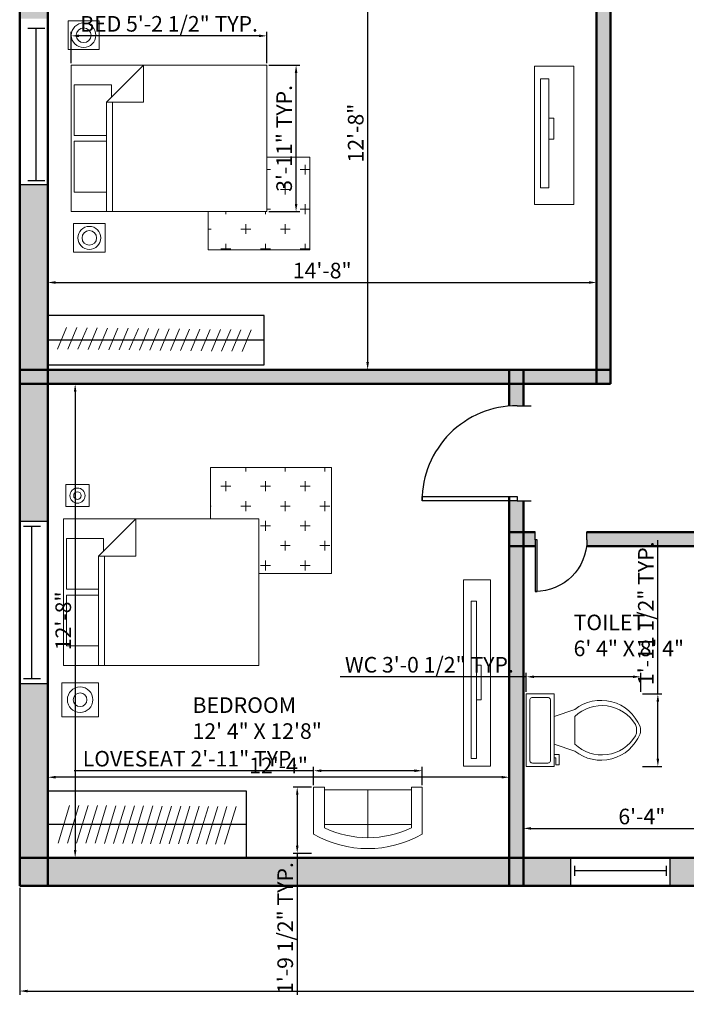
# Model space of a CAD drawing. Units: millimetres. Extents: x 3107 to 3757, y 777 to 1464.
# Tile 1 of 7: x 3110 to 3324, y 824 to 1140. Entities that reach past the tile are written whole.
import ezdxf

# ---------------------------------------------------------------- set-up
doc = ezdxf.new("R2010")
doc.units = ezdxf.units.MM
for name, color, linetype, lineweight in [('A-ANNO-DIMS', 50, 'Continuous', 18), ('A-AREA-IDEN', 160, 'Continuous', 18), ('A-EQPM', 140, 'Continuous', 18), ('A-FLOR-CASE', 140, 'Continuous', 25), ('A-FLOR-CASE-PATT', 140, 'Continuous', 13), ('A-FLOR-FIXT', 140, 'Continuous', 18), ('A-FURN-PATT', 140, 'Continuous', 13), ('A-WALL-PATT', 80, 'Continuous', 13), ('doors', 10, 'Continuous', 25), ('furniture', 140, 'Continuous', 18), ('walls', 80, 'Continuous', 50), ('windows', 30, 'Continuous', 25)]:
    doc.layers.add(name, color=color, linetype=linetype, lineweight=lineweight)
doc.styles.get("Standard").update_dxf_attribs({"font": 'arial.ttf'})
doc.dimstyles.new('ISO-25', dxfattribs={"dimtxt": 5, "dimasz": 2.5, "dimexe": 1.25, "dimexo": 0.625, "dimtad": 1, "dimdec": 0, "dimlunit": 3, "dimtxsty": 'Standard', "dimcen": 2.5, "dimadec": 0, "dimazin": 0, "dimtfac": 1, "dimtdec": 0, "dimtmove": 0, "dimatfit": 3, "dimfxl": 1, "dimarcsym": 0})

# ---------------------------------------------------------------- blocks, each defined once
blk = doc.blocks.new('*U2')
for p, q in [((0, 0), (0, -6)), ((40, 0), (40, -6))]:
    blk.add_line(p, q)
blk.add_lwpolyline([(0, 0), (0, 40), (1.75, 40), (1.75, 0)], close=True)
blk.add_arc((0, 0), 40, 0, 90)
blk = doc.blocks.new('*U4')
for p, q in [((0, 4), (0, 0)), ((36, 4), (36, 0)), ((0, 2), (36, 2))]:
    blk.add_line(p, q)
blk = doc.blocks.new('*U5')
for p, q in [((0, 4), (0, 0)), ((36, 4), (36, 0)), ((0, 2), (36, 2))]:
    blk.add_line(p, q)
blk = doc.blocks.new('Toilet - top')
for p, q in [((9.5, -6), (9.5, -2)), ((-10, -8.5), (-8, -8.5)), ((-10, -9.5), (-10, -8.5)), ((-8, -8.5), (-8, -8)), ((-7, -8), (-7, -9.5)), ((-4, -8), (-6, -14)), ((4, -8), (6, -14)), ((-7, -9.5), (-10, -9.5)), ((4, -14), (-4, -14))]:
    blk.add_line(p, q)
blk.add_lwpolyline([(10.5, -8), (10.5, 0), (-10.5, 0), (-10.5, -8)], close=True)
for points in [[(-9.5, -2), (-9.5, -6)], [(8.5, -1), (-8.5, -1)], [(-8.5, -7), (8.5, -7)]]:
    blk.add_lwpolyline(points)
for centre, radius, start, end in [((-8.62, -1.88), 0.884, 81.8699, 188.1301), ((8.62, -1.88), 0.884, 351.8699, 98.1301), ((-8.62, -6.12), 0.884, 171.8699, 278.1301), ((8.62, -6.12), 0.884, 261.8699, 8.1301), ((3.52, -21.58), 12.17, 141.4691, 247.9714), ((4.2, -21.82), 11.33, 136.3677, 238.9468), ((-3.52, -21.58), 12.17, 292.0284, 38.5307), ((-4.2, -21.82), 11.33, 301.053, 43.6321), ((0, -27.88), 4, 245.7318, 294.2682), ((0, -29), 4, 254.8605, 285.1395)]:
    blk.add_arc(centre, radius, start, end)
blk = doc.blocks.new('Bed - Queen')
for p, q in [((0, -80.00003), (0, 0)), ((0, 0), (59.99999, 0)), ((59.99999, 0), (59.99999, -80.00003)), ((7.99999, -1.2), (28.79998, -1.2)), ((7.99999, -14.4), (7.99999, -1.2)), ((28.79998, -1.2), (28.79998, -14.4)), ((31.19999, -1.2), (51.99999, -1.2)), ((31.19999, -14.4), (31.19999, -1.2)), ((51.99999, -1.2), (51.99999, -16.4)), ((0, -14.4), (44.8, -14.4)), ((59.99999, -29.6), (44.8, -14.4)), ((44.8, -14.4), (44.8, -29.6)), ((44.8, -16.8), (0, -16.8)), ((51.99999, -16.4), (46.79936, -16.4)), ((44.8, -29.6), (59.99999, -29.6)), ((59.99999, -80.00003), (0, -80.00003))]:
    blk.add_line(p, q)
blk = doc.blocks.new('Sofa - Roundback Loveseat 5 ft.')
for p, q in [((0, -32.44198), (0, -5.99998)), ((-24, -33.99998), (-24, -11.46958)), ((-23.9998, -13.38178), (23.99986, -13.38178)), ((24.00004, -33.99998), (24.00004, -11.46958)), ((-24, -32.44198), (24.00004, -32.44198))]:
    blk.add_line(p, q)
for points in [[(-24, -33.99998), (-30, -33.99998), (-30, -7.99998)], [(30.00004, -7.99998), (30.00004, -33.99998), (24.00004, -33.99998)]]:
    blk.add_lwpolyline(points)
for centre, radius, start, end in [((0, -60.24998), 60.24998, 60.13715, 119.8628), ((0, -61.38438), 55.38444, 64.32083, 115.6792)]:
    blk.add_arc(centre, radius, start, end)
blk = doc.blocks.new('*D32')
at = {"layer": 'A-ANNO-DIMS', "color": 0, "lineweight": -2, "transparency": 16777216}
for p, q in [((3119.47, 1056.03), (3119.47, 1054.74)), ((3121.97, 1055.99), (3292.97, 1055.99)), ((3295.47, 1056.03), (3295.47, 1054.74))]:
    blk.add_line(p, q, dxfattribs=at)
at = {"layer": 'A-ANNO-DIMS', "color": 0, "transparency": 16777216}
for points in [[(3121.97, 1056.41), (3121.97, 1055.57), (3119.47, 1055.99)], [(3292.97, 1056.41), (3292.97, 1055.57), (3295.47, 1055.99)]]:
    blk.add_solid(points, dxfattribs=at)
at = {"layer": 'Defpoints', "color": 0, "transparency": 16777216}
for p in [(3119.47, 1056.66), (3295.47, 1056.66), (3295.47, 1055.99)]:
    blk.add_point(p, dxfattribs=at)
at = {"layer": 'A-ANNO-DIMS', "color": 0, "transparency": 16777216, "insert": (3207.47, 1059.17), "char_height": 5, "attachment_point": 5}
blk.add_mtext('14\'-8"', dxfattribs=at)
blk = doc.blocks.new('*D33')
at = {"layer": 'A-ANNO-DIMS', "color": 0, "lineweight": -2, "transparency": 16777216}
for p, q in [((3221.28, 1179.93), (3223.29, 1179.93)), ((3222.04, 1177.43), (3222.04, 1030.43)), ((3221.28, 1027.93), (3223.29, 1027.93))]:
    blk.add_line(p, q, dxfattribs=at)
at = {"layer": 'A-ANNO-DIMS', "color": 0, "transparency": 16777216}
for points in [[(3221.62, 1177.43), (3222.45, 1177.43), (3222.04, 1179.93)], [(3221.62, 1030.43), (3222.45, 1030.43), (3222.04, 1027.93)]]:
    blk.add_solid(points, dxfattribs=at)
at = {"layer": 'Defpoints', "color": 0, "transparency": 16777216}
for p in [(3220.65, 1179.93), (3220.65, 1027.93), (3222.04, 1027.93)]:
    blk.add_point(p, dxfattribs=at)
at = {"layer": 'A-ANNO-DIMS', "color": 0, "transparency": 16777216, "insert": (3218.86, 1103.93), "char_height": 5, "attachment_point": 5, "rotation": 90}
blk.add_mtext('12\'-8"', dxfattribs=at)
blk = doc.blocks.new('*D34')
at = {"layer": 'A-ANNO-DIMS', "color": 0, "lineweight": -2, "transparency": 16777216}
for p, q in [((3119.47, 896.29), (3119.47, 898.5)), ((3264.97, 897.25), (3121.97, 897.25)), ((3267.47, 896.29), (3267.47, 898.5))]:
    blk.add_line(p, q, dxfattribs=at)
at = {"layer": 'A-ANNO-DIMS', "color": 0, "transparency": 16777216}
for points in [[(3121.97, 897.67), (3121.97, 896.84), (3119.47, 897.25)], [(3264.97, 897.67), (3264.97, 896.84), (3267.47, 897.25)]]:
    blk.add_solid(points, dxfattribs=at)
at = {"layer": 'Defpoints', "color": 0, "transparency": 16777216}
for p in [(3119.47, 897.25), (3119.47, 895.66), (3267.47, 895.66)]:
    blk.add_point(p, dxfattribs=at)
at = {"layer": 'A-ANNO-DIMS', "color": 0, "transparency": 16777216, "insert": (3193.47, 900.39), "char_height": 5, "attachment_point": 5}
blk.add_mtext('12\'-4"', dxfattribs=at)
blk = doc.blocks.new('*D35')
at = {"layer": 'A-ANNO-DIMS', "color": 0, "lineweight": -2, "transparency": 16777216}
for p, q in [((3126.83, 1023.43), (3129.5, 1023.43)), ((3128.25, 1020.93), (3128.25, 873.93)), ((3126.83, 871.43), (3129.5, 871.43))]:
    blk.add_line(p, q, dxfattribs=at)
at = {"layer": 'A-ANNO-DIMS', "color": 0, "transparency": 16777216}
for points in [[(3127.84, 1020.93), (3128.67, 1020.93), (3128.25, 1023.43)], [(3127.84, 873.93), (3128.67, 873.93), (3128.25, 871.43)]]:
    blk.add_solid(points, dxfattribs=at)
at = {"layer": 'Defpoints', "color": 0, "transparency": 16777216}
for p in [(3126.21, 1023.43), (3126.21, 871.43), (3128.25, 871.43)]:
    blk.add_point(p, dxfattribs=at)
at = {"layer": 'A-ANNO-DIMS', "color": 0, "transparency": 16777216, "insert": (3125.08, 947.43), "char_height": 5, "attachment_point": 5, "rotation": 90}
blk.add_mtext('12\'-8"', dxfattribs=at)
blk = doc.blocks.new('*D37')
at = {"layer": 'A-ANNO-DIMS', "color": 0, "lineweight": -2, "transparency": 16777216}
for p, q in [((3271.97, 881.46), (3271.97, 882.08)), ((3347.97, 881.46), (3347.97, 882.08)), ((3274.47, 880.83), (3345.47, 880.83))]:
    blk.add_line(p, q, dxfattribs=at)
at = {"layer": 'A-ANNO-DIMS', "color": 0, "transparency": 16777216}
for points in [[(3274.47, 881.25), (3274.47, 880.41), (3271.97, 880.83)], [(3345.47, 881.25), (3345.47, 880.41), (3347.97, 880.83)]]:
    blk.add_solid(points, dxfattribs=at)
at = {"layer": 'Defpoints', "color": 0, "transparency": 16777216}
for p in [(3271.97, 880.83), (3347.97, 880.83), (3347.97, 880.83)]:
    blk.add_point(p, dxfattribs=at)
at = {"layer": 'A-ANNO-DIMS', "color": 0, "transparency": 16777216, "insert": (3309.97, 884.01), "char_height": 5, "attachment_point": 5}
blk.add_mtext('6\'-4"', dxfattribs=at)
blk = doc.blocks.new('*D49')
at = {"layer": 'A-ANNO-DIMS', "color": 0, "lineweight": -2, "transparency": 16777216}
for p, q in [((3127.01, 1126.35), (3127.01, 1136.38)), ((3187.19, 1135.13), (3129.51, 1135.13)), ((3189.69, 1126.35), (3189.69, 1136.38))]:
    blk.add_line(p, q, dxfattribs=at)
at = {"layer": 'A-ANNO-DIMS', "color": 0, "transparency": 16777216}
for points in [[(3129.51, 1135.55), (3129.51, 1134.71), (3127.01, 1135.13)], [(3187.19, 1135.55), (3187.19, 1134.71), (3189.69, 1135.13)]]:
    blk.add_solid(points, dxfattribs=at)
at = {"layer": 'Defpoints', "color": 0, "transparency": 16777216}
for p in [(3127.01, 1135.13), (3127.01, 1125.73), (3189.69, 1125.73)]:
    blk.add_point(p, dxfattribs=at)
at = {"layer": 'A-ANNO-DIMS', "color": 0, "transparency": 16777216, "insert": (3158.35, 1138.34), "char_height": 5, "attachment_point": 5}
blk.add_mtext('BED 5\'-2 1/2" TYP.', dxfattribs=at)
blk = doc.blocks.new('*D50')
at = {"layer": 'A-ANNO-DIMS', "color": 0, "lineweight": -2, "transparency": 16777216}
for p, q in [((3190.32, 1125.73), (3200.34, 1125.73)), ((3199.09, 1081.22), (3199.09, 1123.23)), ((3190.32, 1078.72), (3200.34, 1078.72))]:
    blk.add_line(p, q, dxfattribs=at)
at = {"layer": 'A-ANNO-DIMS', "color": 0, "transparency": 16777216}
for points in [[(3198.68, 1123.23), (3199.51, 1123.23), (3199.09, 1125.73)], [(3198.68, 1081.22), (3199.51, 1081.22), (3199.09, 1078.72)]]:
    blk.add_solid(points, dxfattribs=at)
at = {"layer": 'Defpoints', "color": 0, "transparency": 16777216}
for p in [(3189.69, 1125.73), (3199.09, 1125.73), (3189.69, 1078.72)]:
    blk.add_point(p, dxfattribs=at)
at = {"layer": 'A-ANNO-DIMS', "color": 0, "transparency": 16777216, "insert": (3195.91, 1102.22), "char_height": 5, "attachment_point": 5, "rotation": 90}
blk.add_mtext('3\'-11" TYP.', dxfattribs=at)
blk = doc.blocks.new('*D51')
at = {"layer": 'A-ANNO-DIMS', "color": 0, "lineweight": -2, "transparency": 16777216}
for p, q in [((3272.92, 929.48), (3213.26, 929.48)), ((3272.92, 924.6), (3272.92, 930.73)), ((3307.1, 929.48), (3275.42, 929.48)), ((3309.6, 924.6), (3309.6, 930.73))]:
    blk.add_line(p, q, dxfattribs=at)
at = {"layer": 'A-ANNO-DIMS', "color": 0, "transparency": 16777216}
for points in [[(3275.42, 929.89), (3275.42, 929.06), (3272.92, 929.48)], [(3307.1, 929.89), (3307.1, 929.06), (3309.6, 929.48)]]:
    blk.add_solid(points, dxfattribs=at)
at = {"layer": 'Defpoints', "color": 0, "transparency": 16777216}
for p in [(3272.92, 929.48), (3272.92, 923.97), (3309.6, 923.97)]:
    blk.add_point(p, dxfattribs=at)
at = {"layer": 'A-ANNO-DIMS', "color": 0, "transparency": 16777216, "insert": (3241.84, 932.69), "char_height": 5, "attachment_point": 5}
blk.add_mtext('WC 3\'-0 1/2" TYP.', dxfattribs=at)
blk = doc.blocks.new('*D52')
at = {"layer": 'A-ANNO-DIMS', "color": 0, "lineweight": -2, "transparency": 16777216}
for p, q in [((3315.1, 923.97), (3315.1, 973.27)), ((3310.22, 923.97), (3316.35, 923.97)), ((3315.1, 903.16), (3315.1, 921.47)), ((3310.22, 900.66), (3316.35, 900.66))]:
    blk.add_line(p, q, dxfattribs=at)
at = {"layer": 'A-ANNO-DIMS', "color": 0, "transparency": 16777216}
for points in [[(3314.69, 921.47), (3315.52, 921.47), (3315.1, 923.97)], [(3314.69, 903.16), (3315.52, 903.16), (3315.1, 900.66)]]:
    blk.add_solid(points, dxfattribs=at)
at = {"layer": 'Defpoints', "color": 0, "transparency": 16777216}
for p in [(3309.6, 923.97), (3315.1, 923.97), (3309.6, 900.66)]:
    blk.add_point(p, dxfattribs=at)
at = {"layer": 'A-ANNO-DIMS', "color": 0, "transparency": 16777216, "insert": (3311.89, 949.87), "char_height": 5, "attachment_point": 5, "rotation": 90}
blk.add_mtext('1\'-11 1/2" TYP.', dxfattribs=at)
blk = doc.blocks.new('*D59')
at = {"layer": 'A-ANNO-DIMS', "color": 0, "lineweight": -2, "transparency": 16777216}
for p, q in [((3204.69, 894.74), (3204.69, 900.59)), ((3239.55, 894.74), (3239.55, 900.59)), ((3204.69, 899.34), (3127.98, 899.34)), ((3237.05, 899.34), (3207.19, 899.34))]:
    blk.add_line(p, q, dxfattribs=at)
at = {"layer": 'A-ANNO-DIMS', "color": 0, "transparency": 16777216}
for points in [[(3207.19, 899.76), (3207.19, 898.92), (3204.69, 899.34)], [(3237.05, 899.76), (3237.05, 898.92), (3239.55, 899.34)]]:
    blk.add_solid(points, dxfattribs=at)
at = {"layer": 'Defpoints', "color": 0, "transparency": 16777216}
for p in [(3204.69, 899.34), (3204.69, 894.11), (3239.55, 894.11)]:
    blk.add_point(p, dxfattribs=at)
at = {"layer": 'A-ANNO-DIMS', "color": 0, "transparency": 16777216, "insert": (3165.09, 902.55), "char_height": 5, "attachment_point": 5, "rotation": 360}
blk.add_mtext('LOVESEAT 2\'-11" TYP.', dxfattribs=at)
blk = doc.blocks.new('*D60')
at = {"layer": 'A-ANNO-DIMS', "color": 0, "lineweight": -2, "transparency": 16777216}
for p, q in [((3204.07, 894.11), (3198.21, 894.11)), ((3199.46, 891.61), (3199.46, 875.31)), ((3204.07, 872.81), (3198.21, 872.81)), ((3199.46, 872.81), (3199.46, 827.4))]:
    blk.add_line(p, q, dxfattribs=at)
at = {"layer": 'A-ANNO-DIMS', "color": 0, "transparency": 16777216}
for points in [[(3199.05, 891.61), (3199.88, 891.61), (3199.46, 894.11)], [(3199.05, 875.31), (3199.88, 875.31), (3199.46, 872.81)]]:
    blk.add_solid(points, dxfattribs=at)
at = {"layer": 'Defpoints', "color": 0, "transparency": 16777216}
for p in [(3204.69, 894.11), (3199.46, 872.81), (3204.69, 872.81)]:
    blk.add_point(p, dxfattribs=at)
at = {"layer": 'A-ANNO-DIMS', "color": 0, "transparency": 16777216, "insert": (3196.25, 848.86), "char_height": 5, "attachment_point": 5, "rotation": 90}
blk.add_mtext('1\'-9 1/2" TYP.', dxfattribs=at)
blk = doc.blocks.new('*D69')
at = {"layer": 'A-ANNO-DIMS', "color": 0, "lineweight": -2, "transparency": 16777216}
for p, q in [((3110.47, 861.8), (3110.47, 827.39)), ((3721.97, 861.8), (3721.97, 827.39)), ((3112.97, 828.64), (3719.47, 828.64))]:
    blk.add_line(p, q, dxfattribs=at)
at = {"layer": 'A-ANNO-DIMS', "color": 0, "transparency": 16777216}
for points in [[(3112.97, 829.06), (3112.97, 828.22), (3110.47, 828.64)], [(3719.47, 829.06), (3719.47, 828.22), (3721.97, 828.64)]]:
    blk.add_solid(points, dxfattribs=at)
at = {"layer": 'Defpoints', "color": 0, "transparency": 16777216}
for p in [(3110.47, 862.43), (3721.97, 862.43), (3721.97, 828.64)]:
    blk.add_point(p, dxfattribs=at)
at = {"layer": 'A-ANNO-DIMS', "color": 0, "transparency": 16777216, "insert": (3416.22, 831.85), "char_height": 5, "attachment_point": 5}
blk.add_mtext('50\'-11 1/2"', dxfattribs=at)

msp = doc.modelspace()

# ---------------------------------------------------------------- hatches: boundary and pattern name
at = {"layer": 'A-FLOR-CASE-PATT'}
h = msp.add_hatch(dxfattribs=at)
h.set_pattern_fill('ANSI31', color=256, scale=0.960855, angle=22.188, style=0)
h.paths.add_polyline_path([(3120.7, 1034.66), (3123.99, 1034.62), (3130.57, 1034.53), (3166.78, 1034.07), (3176.66, 1033.94), (3183.24, 1033.85), (3186.14, 1040.76), (3123.6, 1041.57)])
h = msp.add_hatch(dxfattribs=at)
h.set_pattern_fill('ANSI31', color=256, scale=0.895394, angle=27.967, style=0)
h.paths.add_polyline_path([(3120.31, 876.16), (3126.24, 876.12), (3155.91, 875.91), (3161.84, 875.87), (3176.68, 875.76), (3180.38, 887.84), (3150.71, 888.05), (3147.74, 888.07), (3124.01, 888.24)])
at = {"layer": 'A-FURN-PATT'}
h = msp.add_hatch(dxfattribs=at)
h.set_pattern_fill('CROSS', color=256)
h.paths.add_polyline_path([(3203.54, 1096.17), (3189.69, 1096.17), (3189.69, 1078.72), (3170.92, 1078.72), (3170.92, 1066.5), (3203.54, 1066.5)])
h = msp.add_hatch(dxfattribs=at)
h.set_pattern_fill('CROSS', color=256)
h.paths.add_polyline_path([(3171.7, 996.6), (3171.7, 980.14), (3187.18, 980.14), (3187.18, 962.6), (3210.42, 962.6), (3210.42, 996.6)])
at = {"layer": 'A-WALL-PATT'}
h = msp.add_hatch(color=256, dxfattribs=at)
h.dxf.hatch_style = 1
h.paths.add_polyline_path([(3119.47, 1087.39), (3110.47, 1087.39), (3110.47, 1027.93), (3119.47, 1027.93)])
h.paths.add_polyline_path([(3119.47, 1027.93), (3110.47, 1027.93), (3110.47, 1023.43), (3119.47, 1023.43)])
h.paths.add_polyline_path([(3267.47, 1027.93), (3119.47, 1027.93), (3119.47, 1023.43), (3267.47, 1023.43)])
h.paths.add_polyline_path([(3119.47, 1023.43), (3110.47, 1023.43), (3110.47, 979.44), (3119.47, 979.44)])
h.paths.add_polyline_path([(3299.97, 1179.93), (3295.47, 1179.93), (3295.47, 1027.93), (3299.97, 1027.93)])
h.paths.add_polyline_path([(3295.47, 1027.93), (3271.97, 1027.93), (3271.97, 1023.43), (3295.47, 1023.43)])
h.paths.add_polyline_path([(3271.97, 1027.93), (3267.47, 1027.93), (3267.47, 1023.43), (3271.97, 1023.43)])
h.paths.add_polyline_path([(3299.97, 1027.93), (3295.47, 1027.93), (3295.47, 1023.43), (3299.97, 1023.43)])
h.paths.add_polyline_path([(3299.97, 1184.43), (3295.47, 1184.43), (3295.47, 1179.93), (3299.97, 1179.93)])
h.paths.add_polyline_path([(3295.47, 1184.43), (3288.38, 1184.43), (3288.38, 1182.47), (3288.38, 1179.93), (3295.47, 1179.93)])
h.paths.add_polyline_path([(3352.47, 1179.93), (3347.97, 1179.93), (3347.97, 1027.93), (3352.47, 1027.93)])
h.paths.add_polyline_path([(3352.47, 1184.43), (3347.97, 1184.43), (3347.97, 1179.93), (3352.47, 1179.93)])
h.paths.add_polyline_path([(3464.47, 1184.43), (3352.47, 1184.43), (3352.47, 1179.93), (3464.47, 1179.93)])
h.paths.add_polyline_path([(3468.97, 1288.93), (3464.47, 1288.93), (3464.47, 1184.43), (3468.97, 1184.43)])
h.paths.add_polyline_path([(3468.97, 1184.43), (3464.47, 1184.43), (3464.47, 1179.93), (3468.97, 1179.93)])
h.paths.add_polyline_path([(3195.97, 1248.43), (3191.47, 1248.43), (3191.47, 1184.43), (3195.97, 1184.43)])
h.paths.add_polyline_path([(3195.97, 1184.43), (3191.47, 1184.43), (3191.47, 1179.93), (3195.97, 1179.93)])
h.paths.add_polyline_path([(3191.47, 1184.43), (3183.28, 1184.43), (3183.28, 1181.58), (3183.28, 1179.93), (3191.47, 1179.93)])
h.paths.add_polyline_path([(3243.97, 1184.43), (3195.97, 1184.43), (3195.97, 1179.93), (3243.97, 1179.93)])
h.paths.add_polyline_path([(3257.91, 1182.47), (3257.91, 1184.43), (3248.47, 1184.43), (3248.47, 1179.93), (3258.02, 1179.93, -0.020891)])
h.paths.add_polyline_path([(3248.47, 1184.43), (3243.97, 1184.43), (3243.97, 1179.93), (3248.47, 1179.93)])
h.paths.add_polyline_path([(3248.47, 1189.24), (3247.51, 1189.24), (3243.97, 1189.24), (3243.97, 1184.43), (3248.47, 1184.43)])
h.paths.add_polyline_path([(3166.87, 1184.43), (3119.47, 1184.43), (3119.47, 1179.93), (3166.63, 1179.93), (3166.63, 1181.58, -0.042981)])
h.paths.add_polyline_path([(3119.47, 1184.43), (3110.47, 1184.43), (3110.47, 1179.93), (3119.47, 1179.93)])
h.paths.add_polyline_path([(3119.47, 1248.43), (3110.47, 1248.43), (3110.47, 1184.43), (3119.47, 1184.43)])
h.paths.add_polyline_path([(3119.47, 1179.93), (3110.47, 1179.93), (3110.47, 1140.65), (3119.47, 1140.65)])
h.paths.add_polyline_path([(3119.47, 1288.93), (3110.47, 1288.93), (3110.47, 1252.93), (3119.47, 1252.93)])
h.paths.add_polyline_path([(3119.47, 1252.93), (3110.47, 1252.93), (3110.47, 1248.43), (3119.47, 1248.43)])
h.paths.add_polyline_path([(3191.47, 1252.93), (3119.47, 1252.93), (3119.47, 1248.43), (3191.47, 1248.43)])
h.paths.add_polyline_path([(3195.97, 1288.93), (3191.47, 1288.93), (3191.47, 1252.93), (3195.97, 1252.93)])
h.paths.add_polyline_path([(3195.97, 1252.93), (3191.47, 1252.93), (3191.47, 1248.43), (3195.97, 1248.43)])
h.paths.add_polyline_path([(3248.47, 1293.43), (3243.97, 1293.43), (3243.97, 1288.93), (3248.47, 1288.93)])
h.paths.add_polyline_path([(3243.97, 1293.43), (3195.97, 1293.43), (3195.97, 1288.93), (3243.97, 1288.93)])
h.paths.add_polyline_path([(3303.47, 1293.43), (3248.47, 1293.43), (3248.47, 1288.93), (3303.47, 1288.93)])
h.paths.add_polyline_path([(3248.47, 1288.93), (3243.97, 1288.93), (3243.97, 1205.51, -0.053712), (3247.51, 1205.89), (3248.47, 1205.89)])
h.paths.add_polyline_path([(3191.47, 1293.43), (3119.47, 1293.43), (3119.47, 1288.93), (3191.47, 1288.93)])
h.paths.add_polyline_path([(3119.47, 1293.43), (3110.47, 1293.43), (3110.47, 1288.93), (3119.47, 1288.93)])
h.paths.add_polyline_path([(3119.47, 1322.96, -0.065064), (3111.64, 1321.93), (3110.47, 1321.93), (3110.47, 1293.43), (3119.47, 1293.43)])
h.paths.add_polyline_path([(3195.97, 1293.43), (3191.47, 1293.43), (3191.47, 1288.93), (3195.97, 1288.93)])
h.paths.add_polyline_path([(3119.47, 1450.43), (3110.47, 1450.43), (3110.47, 1441.43), (3119.47, 1441.43)])
h.paths.add_polyline_path([(3119.47, 1441.43), (3110.47, 1441.43), (3110.47, 1352.4), (3111.64, 1352.4), (3119.47, 1352.4)])
h.paths.add_polyline_path([(3176.58, 1450.43), (3119.47, 1450.43), (3119.47, 1441.43), (3176.58, 1441.43)])
h.paths.add_polyline_path([(3323.19, 1450.43), (3307.97, 1450.43), (3307.97, 1441.43), (3323.19, 1441.43)])
h.paths.add_polyline_path([(3307.97, 1450.43), (3303.47, 1450.43), (3303.47, 1441.43), (3307.97, 1441.43)])
h.paths.add_polyline_path([(3303.47, 1450.43), (3229.4, 1450.43), (3229.4, 1441.43), (3303.47, 1441.43)])
h.paths.add_polyline_path([(3307.97, 1441.43), (3303.47, 1441.43), (3303.47, 1363.43), (3307.97, 1363.43)])
h.paths.add_polyline_path([(3307.97, 1363.43), (3303.47, 1363.43), (3303.47, 1358.93), (3307.97, 1358.93)])
h.paths.add_polyline_path([(3307.97, 1358.93), (3303.47, 1358.93), (3303.47, 1342.3), (3305.5, 1342.3, -0.037178), (3307.97, 1342.12)])
h.paths.add_polyline_path([(3379.97, 1363.43), (3307.97, 1363.43), (3307.97, 1358.93), (3379.97, 1358.93)])
h.paths.add_polyline_path([(3384.47, 1393.61), (3383.04, 1393.61), (3379.97, 1393.61), (3379.97, 1363.43), (3384.47, 1363.43)])
h.paths.add_polyline_path([(3384.47, 1363.43), (3379.97, 1363.43), (3379.97, 1358.93), (3384.47, 1358.93)])
h.paths.add_polyline_path([(3384.47, 1358.93), (3379.97, 1358.93), (3379.97, 1293.43), (3384.47, 1293.43)])
h.paths.add_polyline_path([(3384.47, 1441.43), (3379.97, 1441.43), (3379.97, 1409.98, -0.046389), (3383.04, 1410.27), (3384.47, 1410.27)])
h.paths.add_polyline_path([(3384.47, 1450.43), (3379.97, 1450.43), (3379.97, 1441.43), (3384.47, 1441.43)])
h.paths.add_polyline_path([(3379.97, 1450.43), (3357.18, 1450.43), (3357.18, 1441.43), (3379.97, 1441.43)])
h.paths.add_polyline_path([(3432.79, 1450.43), (3384.47, 1450.43), (3384.47, 1441.43), (3432.79, 1441.43)])
h.paths.add_polyline_path([(3540.47, 1450.43), (3484.18, 1450.43), (3484.18, 1441.43), (3540.47, 1441.43)])
h.paths.add_polyline_path([(3544.97, 1450.43), (3540.47, 1450.43), (3540.47, 1441.43), (3544.97, 1441.43)])
h.paths.add_polyline_path([(3544.97, 1441.43), (3540.47, 1441.43), (3540.47, 1293.43), (3544.97, 1293.43)])
h.paths.add_polyline_path([(3590.83, 1450.43), (3544.97, 1450.43), (3544.97, 1441.43), (3590.83, 1441.43)])
h.paths.add_polyline_path([(3712.97, 1450.43), (3645.62, 1450.43), (3645.62, 1441.43), (3712.97, 1441.43)])
h.paths.add_polyline_path([(3721.97, 1441.43), (3712.97, 1441.43), (3712.97, 1288.93), (3712.97, 1184.43), (3721.97, 1184.43), (3721.97, 1288.93)])
h.paths.add_polyline_path([(3721.97, 1450.43), (3712.97, 1450.43), (3712.97, 1441.43), (3721.97, 1441.43)])
h.paths.add_polyline_path([(3712.97, 1184.43), (3658.24, 1184.43), (3658.24, 1183.15), (3658.24, 1179.93), (3712.97, 1179.93)])
h.paths.add_polyline_path([(3721.97, 1184.43), (3712.97, 1184.43), (3712.97, 1179.93), (3721.97, 1179.93)])
h.paths.add_polyline_path([(3597.32, 1183.15), (3597.32, 1184.43), (3544.97, 1184.43), (3544.97, 1179.93), (3597.32, 1179.93)])
h.paths.add_polyline_path([(3544.97, 1184.43), (3540.47, 1184.43), (3540.47, 1179.93), (3544.97, 1179.93)])
h.paths.add_polyline_path([(3544.97, 1179.93), (3540.47, 1179.93), (3540.47, 1143.69), (3543.65, 1143.69), (3544.97, 1143.69)])
h.paths.add_polyline_path([(3721.97, 1179.93), (3712.97, 1179.93), (3712.97, 1006.22), (3712.97, 871.43), (3721.97, 871.43), (3721.97, 1006.22)])
h.paths.add_polyline_path([(3468.97, 1293.43), (3464.47, 1293.43), (3464.47, 1288.93), (3468.97, 1288.93)])
h.paths.add_polyline_path([(3540.47, 1293.43), (3468.97, 1293.43), (3468.97, 1288.93), (3540.47, 1288.93)])
h.paths.add_polyline_path([(3544.97, 1293.43), (3540.47, 1293.43), (3540.47, 1288.93), (3544.97, 1288.93)])
h.paths.add_polyline_path([(3464.47, 1293.43), (3417.83, 1293.43, -0.015057), (3417.88, 1291.6), (3417.88, 1288.93), (3464.47, 1288.93)])
h.paths.add_polyline_path([(3379.97, 1293.43), (3307.97, 1293.43), (3307.97, 1288.93), (3379.97, 1288.93)])
h.paths.add_polyline_path([(3307.97, 1325.65), (3305.5, 1325.65), (3303.47, 1325.65), (3303.47, 1293.43), (3307.97, 1293.43)])
h.paths.add_polyline_path([(3307.97, 1293.43), (3303.47, 1293.43), (3303.47, 1288.93), (3307.97, 1288.93)])
h.paths.add_polyline_path([(3384.47, 1293.43), (3379.97, 1293.43), (3379.97, 1288.93), (3384.47, 1288.93)])
h.paths.add_polyline_path([(3387.42, 1291.6), (3387.42, 1293.43), (3384.47, 1293.43), (3384.47, 1288.93), (3387.42, 1288.93)])
h.paths.add_polyline_path([(3119.47, 927.28), (3110.47, 927.28), (3110.47, 871.43), (3119.47, 871.43)])
h.paths.add_polyline_path([(3119.47, 871.43), (3110.47, 871.43), (3110.47, 862.43), (3119.47, 862.43)])
h.paths.add_polyline_path([(3267.47, 871.43), (3119.47, 871.43), (3119.47, 862.43), (3267.47, 862.43)])
h.paths.add_polyline_path([(3271.97, 971.43), (3267.47, 971.43), (3267.47, 871.43), (3271.97, 871.43)])
h.paths.add_polyline_path([(3271.97, 871.43), (3267.47, 871.43), (3267.47, 862.43), (3271.97, 862.43)])
h.paths.add_polyline_path([(3287.13, 871.43), (3271.97, 871.43), (3271.97, 862.43), (3287.13, 862.43)])
h.paths.add_polyline_path([(3347.97, 871.43), (3318.96, 871.43), (3318.96, 862.43), (3347.97, 862.43)])
h.paths.add_polyline_path([(3352.47, 971.43), (3347.97, 971.43), (3347.97, 871.43), (3352.47, 871.43)])
h.paths.add_polyline_path([(3352.47, 871.43), (3347.97, 871.43), (3347.97, 862.43), (3352.47, 862.43)])
h.paths.add_polyline_path([(3375.96, 871.43), (3352.47, 871.43), (3352.47, 862.43), (3375.96, 862.43)])
h.paths.add_polyline_path([(3352.47, 975.93), (3347.97, 975.93), (3347.97, 971.43), (3352.47, 971.43)])
h.paths.add_polyline_path([(3352.47, 986.27, -0.01722), (3350.37, 986.2), (3347.97, 986.2), (3347.97, 975.93), (3352.47, 975.93)])
h.paths.add_polyline_path([(3347.97, 975.93), (3292.38, 975.93), (3292.38, 973.47, -0.030785), (3292.25, 971.43), (3347.97, 971.43)])
h.paths.add_polyline_path([(3271.97, 985.98), (3269.95, 985.98), (3267.47, 985.98), (3267.47, 975.93), (3271.97, 975.93)])
h.paths.add_polyline_path([(3271.97, 975.93), (3267.47, 975.93), (3267.47, 971.43), (3271.97, 971.43)])
h.paths.add_polyline_path([(3275.72, 975.93), (3271.97, 975.93), (3271.97, 971.43), (3275.72, 971.43), (3275.72, 973.47)])
h.paths.add_polyline_path([(3271.97, 1023.43), (3267.47, 1023.43), (3267.47, 1016.34, -0.020418), (3269.95, 1016.44), (3271.97, 1016.44)])
h.paths.add_polyline_path([(3352.47, 1023.43), (3347.97, 1023.43), (3347.97, 1016.67), (3350.37, 1016.67), (3352.47, 1016.67)])
h.paths.add_polyline_path([(3352.47, 1027.93), (3347.97, 1027.93), (3347.97, 1023.43), (3352.47, 1023.43)])
h.paths.add_polyline_path([(3476.47, 1027.93), (3352.47, 1027.93), (3352.47, 1023.43), (3476.47, 1023.43)])
h.paths.add_polyline_path([(3540.47, 1027.93), (3480.97, 1027.93), (3480.97, 1023.43), (3540.47, 1023.43)])
h.paths.add_polyline_path([(3480.97, 1027.93), (3476.47, 1027.93), (3476.47, 1023.43), (3480.97, 1023.43)])
h.paths.add_polyline_path([(3480.97, 1023.43), (3476.47, 1023.43), (3476.47, 871.43), (3480.97, 871.43)])
h.paths.add_polyline_path([(3476.47, 871.43), (3429.88, 871.43), (3429.88, 862.43), (3476.47, 862.43)])
h.paths.add_polyline_path([(3480.97, 871.43), (3476.47, 871.43), (3476.47, 862.43), (3480.97, 862.43)])
h.paths.add_polyline_path([(3493.81, 871.43), (3480.97, 871.43), (3480.97, 862.43), (3493.81, 862.43)])
h.paths.add_polyline_path([(3712.97, 871.43), (3525.61, 871.43), (3525.61, 862.43), (3712.97, 862.43)])
h.paths.add_polyline_path([(3721.97, 871.43), (3712.97, 871.43), (3712.97, 862.43), (3721.97, 862.43)])

# ---------------------------------------------------------------- linework, layer by layer
at = {"layer": 'A-EQPM'}
for points in [[(3275.55, 1125.39), (3288.18, 1125.39), (3288.18, 1081.06), (3275.55, 1081.06)], [(3277.46, 1121.35), (3280.17, 1121.35), (3280.17, 1086.41), (3277.46, 1086.41)], [(3280.17, 1108.69), (3281.76, 1108.69), (3281.76, 1101.93), (3280.17, 1101.93)], [(3261.45, 960.59), (3252.81, 960.59), (3252.81, 900.76), (3261.45, 900.76)], [(3255.24, 953.73), (3256.9, 953.73), (3256.9, 903.22), (3255.24, 903.22)], [(3256.9, 933.26), (3258.45, 933.26), (3258.45, 922.1), (3256.9, 922.1)]]:
    msp.add_lwpolyline(points, close=True, dxfattribs=at)
at = {"layer": 'A-FLOR-CASE'}
for p, q in [((3188.84, 1037.52), (3119.47, 1037.52)), ((3183.17, 882.11), (3119.47, 882.11))]:
    msp.add_line(p, q, dxfattribs=at)
for points in [[(3119.47, 1029.59), (3188.84, 1029.59), (3188.84, 1045.44), (3119.47, 1045.44)], [(3119.47, 871.43), (3183.17, 871.43), (3183.17, 892.78), (3119.47, 892.78)]]:
    msp.add_lwpolyline(points, close=True, dxfattribs=at)
at = {"layer": 'furniture'}
for p, q in [((3189.69, 1096.17), (3203.54, 1096.17)), ((3203.54, 1096.17), (3203.54, 1066.5)), ((3170.92, 1066.5), (3170.92, 1078.72)), ((3203.54, 1066.5), (3170.92, 1066.5)), ((3210.42, 996.6), (3171.7, 996.6)), ((3171.7, 996.6), (3171.7, 980.14)), ((3210.42, 962.6), (3210.42, 996.6)), ((3187.18, 962.6), (3210.42, 962.6))]:
    msp.add_line(p, q, dxfattribs=at)
for points in [[(3126.01, 1130.71), (3135.92, 1130.71), (3135.92, 1139.94), (3126.01, 1139.94)], [(3127.74, 1074.87), (3137.85, 1074.87), (3137.85, 1065.74), (3127.74, 1065.74)], [(3125.23, 984.07), (3132.76, 984.07), (3132.76, 991.15), (3125.23, 991.15)], [(3123.93, 927.57), (3135.74, 927.57), (3135.74, 916.68), (3123.93, 916.68)]]:
    msp.add_lwpolyline(points, close=True, dxfattribs=at)
for centre, radius in [((3130.96, 1135.32), 3.94), ((3130.96, 1135.32), 2.37), ((3132.79, 1070.31), 3.68), ((3132.79, 1070.31), 2.34), ((3128.99, 987.61), 2.43), ((3128.99, 987.61), 1.21), ((3129.83, 922.12), 4.09), ((3129.83, 922.12), 2.21)]:
    msp.add_circle(centre, radius, dxfattribs=at)
at = {"layer": 'walls'}
for p, q in [((3110.47, 1321.93), (3110.47, 862.43)), ((3119.47, 1322.96), (3119.47, 862.43)), ((3295.47, 1184.43), (3295.47, 1023.43)), ((3299.97, 1184.43), (3299.97, 1023.43)), ((3110.47, 1027.93), (3299.97, 1027.93)), ((3267.47, 1027.93), (3267.47, 1016.34)), ((3271.97, 1027.93), (3271.97, 1016.44)), ((3110.47, 1023.43), (3299.97, 1023.43)), ((3267.47, 987.31), (3267.47, 862.43)), ((3271.97, 985.98), (3271.97, 862.43)), ((3267.47, 975.93), (3275.72, 975.93)), ((3292.38, 975.93), (3352.47, 975.93)), ((3267.47, 971.43), (3275.72, 971.43)), ((3292.25, 971.43), (3352.47, 971.43)), ((3110.47, 871.43), (3721.97, 871.43)), ((3110.47, 862.43), (3721.97, 862.43))]:
    msp.add_line(p, q, dxfattribs=at)
at = {"layer": 'windows'}
for p, q in [((3110.47, 1087.39), (3119.47, 1087.39)), ((3110.47, 979.44), (3119.47, 979.44)), ((3110.47, 927.28), (3119.47, 927.28)), ((3287.13, 871.43), (3287.13, 862.43)), ((3318.96, 871.43), (3318.96, 862.43))]:
    msp.add_line(p, q, dxfattribs=at)

# ---------------------------------------------------------------- block references
at = {"layer": 'A-FLOR-FIXT', "xscale": 1.109949414103811, "yscale": 1.109949414103811, "zscale": 1.109949414103811, "rotation": 90}
msp.add_blockref('Toilet - top', (3272.92, 912.32), dxfattribs=at)
at = {"layer": 'doors'}
for p, xscale, yscale, zscale, rotation in [((3269.95, 985.98), 0.7615706373352984, 0.7615706373352984, 0.7615706373352984, 89.99999999999996), ((3275.72, 973.47), -0.4163085604342208, 0.4163085604342208, 0.4163085604342208, 180)]:
    msp.add_blockref('*U2', p, dxfattribs=dict(at, xscale=xscale, yscale=yscale, zscale=zscale, rotation=rotation))
at = {"layer": 'furniture'}
for name, p, xscale, yscale, zscale, rotation in [('Bed - Queen', (3127.01, 1078.72), 0.7835133119924312, 0.7835133119924312, 0.7835133119924312, 90.00000000000317), ('Bed - Queen', (3124.5, 933.13), 0.7835133119924312, 0.7835133119924312, 0.7835133119924312, 90.00000000000317), ('Sofa - Roundback Loveseat 5 ft.', (3222.12, 874.36), 0.5809767439628069, 0.5809767439628069, 0.5809767439628069, 179.9999691995332)]:
    msp.add_blockref(name, p, dxfattribs=dict(at, xscale=xscale, yscale=yscale, zscale=zscale, rotation=rotation))
at = {"layer": 'windows'}
for name, p, xscale, yscale, zscale, rotation in [('*U4', (3118.49, 1088.67), 1.357941570966636, 1.357941570966636, 1.357941570966636, 90), ('*U4', (3117.11, 928.95), 1.357941570966636, 1.357941570966636, 1.357941570966636, 90), ('*U5', (3317.87, 868.85), 0.8150463067894532, 0.8150463067894532, 0.8150463067894532, 180)]:
    msp.add_blockref(name, p, dxfattribs=dict(at, xscale=xscale, yscale=yscale, zscale=zscale, rotation=rotation))

# ---------------------------------------------------------------- texts
at = {"layer": 'A-AREA-IDEN', "char_height": 5, "attachment_point": 1}
for s, width, insert in [('TOILET\\P6\' 4" X 8\' 4"', 49.8149, (3288.08, 949.42)), ('BEDROOM\\P12\' 4" X 12\'8"', 50.5595, (3165.88, 922.89))]:
    msp.add_mtext_dynamic_manual_height_columns(s, width=width, gutter_width=12.5, heights=[0], dxfattribs=dict(at, insert=insert))

# ---------------------------------------------------------------- dimensions: what is measured, and where the dimension line sits
at = {"layer": 'A-ANNO-DIMS'}
for base, p1, p2, picture, middle in [((3222.04, 1027.93), (3220.65, 1179.93), (3220.65, 1027.93), '*D33', (3218.86, 1103.93)), ((3128.25, 871.43), (3126.21, 1023.43), (3126.21, 871.43), '*D35', (3125.08, 947.43))]:
    dim = msp.add_linear_dim(base=base, p1=p1, p2=p2, angle=90, dimstyle='ISO-25', override={"dimclrd": 0, "dimclre": 0, "dimclrt": 0}, dxfattribs=at)
    dim.commit()
    dim.dimension.update_dxf_attribs({"geometry": picture, "text_midpoint": middle})
for base, p1, p2, angle, text, picture, middle in [((3127.01, 1135.13), (3189.69, 1125.73), (3127.01, 1125.73), 180, 'BED <> TYP.', '*D49', (3158.35, 1138.34)), ((3199.09, 1125.73), (3189.69, 1078.72), (3189.69, 1125.73), 90, '<> TYP.', '*D50', (3195.91, 1102.22)), ((3315.1, 923.97), (3309.6, 900.66), (3309.6, 923.97), 90, '<> TYP.', '*D52', (3311.89, 949.87)), ((3272.92, 929.48), (3309.6, 923.97), (3272.92, 923.97), 180, 'WC <> TYP.', '*D51', (3241.84, 932.69)), ((3204.69, 899.34), (3239.55, 894.11), (3204.69, 894.11), 180, 'LOVESEAT <> TYP.', '*D59', (3165.09, 902.55)), ((3199.46, 872.81), (3204.69, 894.11), (3204.69, 872.81), 270, '<> TYP.', '*D60', (3196.25, 848.86))]:
    dim = msp.add_linear_dim(base=base, p1=p1, p2=p2, angle=angle, text=text, dimstyle='ISO-25', override={"dimdec": 1, "dimlfac": 1, "dimrnd": 0, "dimzin": 1, "dimdsep": 46, "dimlunit": 4, "dimfrac": 2}, dxfattribs=at)
    dim.commit()
    dim.dimension.update_dxf_attribs({"geometry": picture, "text_midpoint": middle})
for base, p1, p2, override, picture, middle in [((3295.47, 1055.99), (3119.47, 1056.66), (3295.47, 1056.66), {"dimclrd": 0, "dimclre": 0, "dimclrt": 0}, '*D32', (3207.47, 1059.17)), ((3119.47, 897.25), (3267.47, 895.66), (3119.47, 895.66), {"dimclrd": 0, "dimclre": 0, "dimclrt": 0}, '*D34', (3193.47, 900.39)), ((3347.97, 880.83), (3271.97, 880.83), (3347.97, 880.83), {"dimclrd": 0, "dimclre": 0, "dimclrt": 0}, '*D37', (3309.97, 884.01)), ((3721.97, 828.64), (3110.47, 862.43), (3721.97, 862.43), {"dimdec": 1, "dimlfac": 1, "dimrnd": 0, "dimzin": 1, "dimdsep": 46, "dimlunit": 4, "dimfrac": 2}, '*D69', (3416.22, 831.85))]:
    dim = msp.add_linear_dim(base=base, p1=p1, p2=p2, dimstyle='ISO-25', override=override, dxfattribs=at)
    dim.commit()
    dim.dimension.update_dxf_attribs({"geometry": picture, "text_midpoint": middle})

doc.saveas('drawing.dxf')
